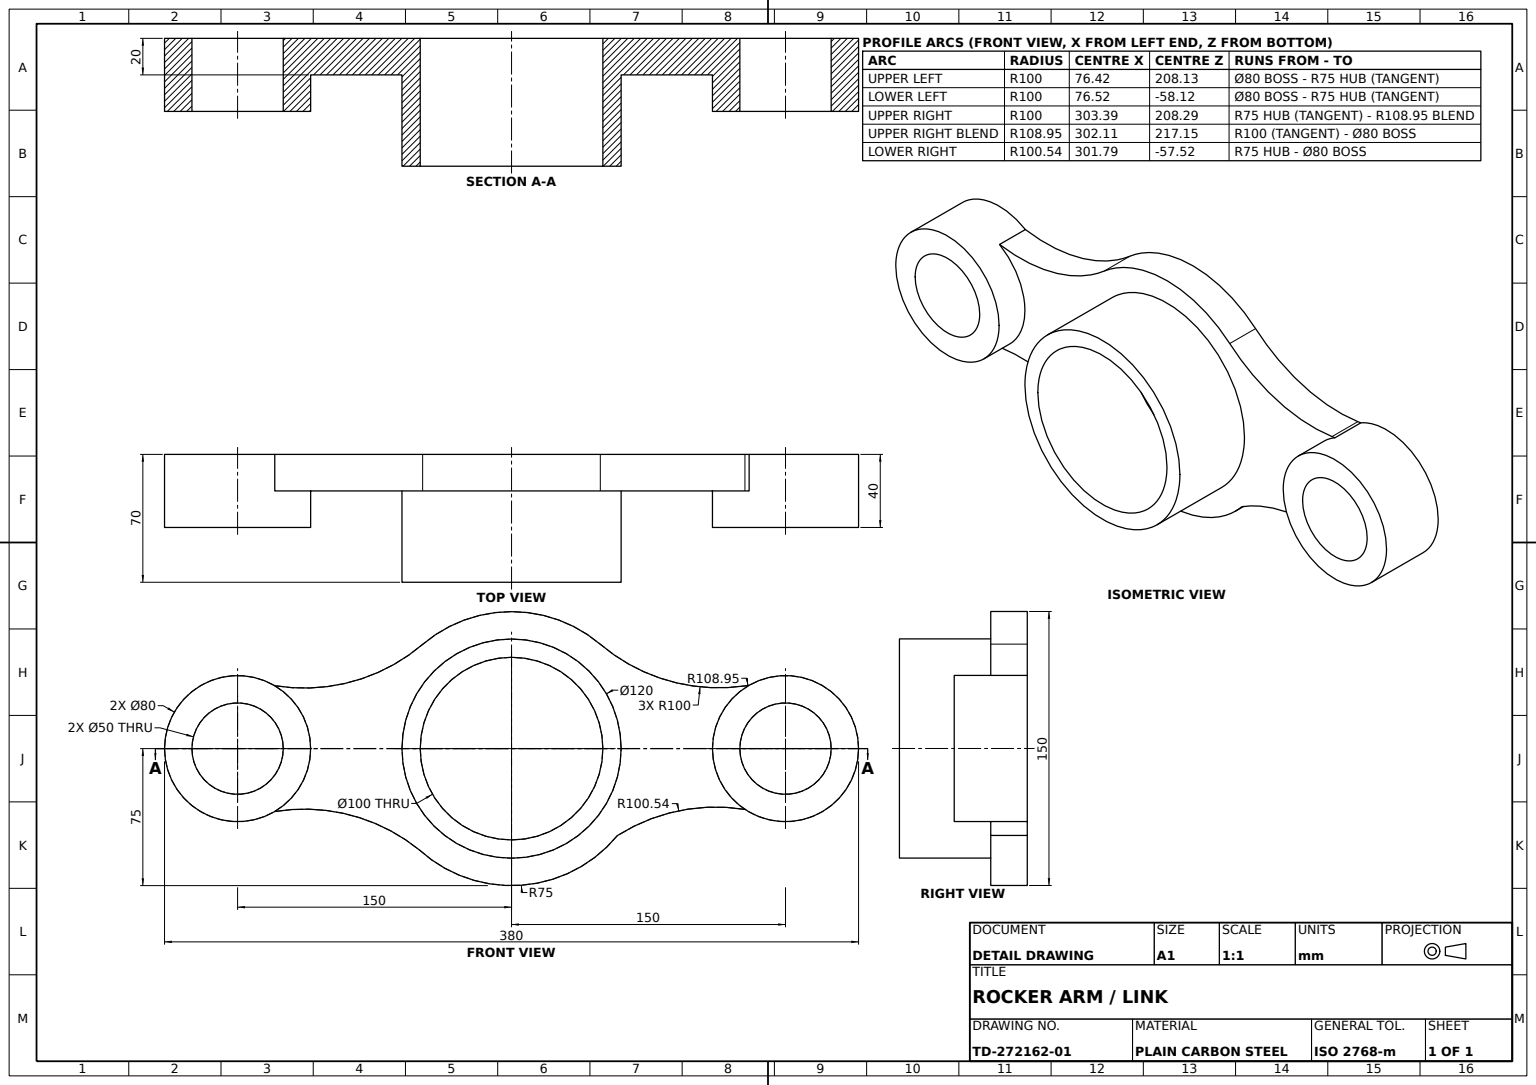
SolidWorks part; units mm, degrees
material "Plain Carbon Steel"
ref_plane "Front Plane" through (0, 0, 0) normal (0, 0, 1) x (1, 0, 0)
ref_plane "Top Plane" through (0, 0, 0) normal (0, 1, 0) x (1, 0, 0)
ref_plane "Right Plane" through (0, 0, 0) normal (1, 0, 0) x (0, 0, -1)
sketch "Link Profile Sketch" plane through (0, 0, 0) normal (0, 0, 1) x (1, 0, 0)
  arc A1 (-129.6423, 34.432) -> (-129.6423, -34.432) centre (-150, 0) ccw
  arc A2 (127.7843, -33.2635) -> (130.0893, 34.6924) centre (150, 0) ccw
  arc A3 (-150, 40) -> (-147.9847, 39.2383) centre (-111.3927, 139.1034) ccw
  arc A4 (-50.5482, -55.4065) -> (57.9498, -47.6111) centre (0, 0) ccw
  arc A5 (127.7843, 34.332) -> (130.0893, 34.6924) centre (112.1066, 142.1518) ccw
  arc A6 (-129.6423, -34.432) -> (-50.5482, -55.4065) centre (-113.4841, -133.1179) cw
  arc A7 (48.5979, 57.1249) -> (-48.6772, 57.0573) centre (0, 0) ccw
  arc A8 (127.7843, 34.332) -> (48.5979, 57.1249) centre (113.395, 133.2913) cw
  arc A9 (-129.6423, 34.432) -> (-48.6772, 57.0573) centre (-113.5801, 133.1336) ccw
  arc A10 (127.7843, -33.2635) -> (57.9498, -47.6111) centre (111.7861, -132.5225) ccw
  arc A11 (48.5979, 57.1249) -> (-48.6772, 57.0573) centre (0, 0) ccw
  point P20 (57.9498, 47.6111)
  dimension "D1" = 150
  dimension "D2" = 80
  dimension "D3" = 80
  dimension "D4" = 100
  dimension "D5" = 100
  dimension "D6" = 100
  dimension "D7" = 40
  dimension "D8" = 106.358
  dimension "D9" = 75
  dimension "D10" = 108.9536
  dimension "D11" = 100.54
  dimension "D12" = 19.9107
  dimension "D13" = 22.2157
  dimension "D14" = 36.605
  dimension "D15" = 198.6772
  dimension "D16" = 200.5482
  dimension "D17" = 261.3927
extrude "Link Plate" add sketch "Link Profile Sketch" along normal blind 20
sketch "Center Boss Sketch" plane through (0, 0, 20) normal (0, 0, 1) x (1, 0, 0)
  circle A0 centre (0, 0) radius 60
  dimension "D1" = 120
  dimension "D2" = 120
extrude "Center Boss Ø120" add sketch "Center Boss Sketch" along normal blind 50
sketch "Center Bore Sketch" plane through (0, 0, 70) normal (0, 0, 1) x (1, 0, 0)
  circle A0 centre (0, 0) radius 50
  dimension "D1" = 100
  dimension "D2" = 100
extrude "Center Bore Ø100" cut sketch "Center Bore Sketch" against normal blind 70
sketch "End Boss A Sketch" plane through (0, 0, 20) normal (0, 0, 1) x (1, 0, 0)
  circle A0 centre (-150, 0) radius 40
  dimension "D1" = 80
  dimension "D2" = 80
extrude "End Boss A Ø80" add sketch "End Boss A Sketch" along normal blind 20
sketch "End Boss B Sketch" plane through (0, 0, 20) normal (0, 0, 1) x (1, 0, 0)
  circle A0 centre (150, 0) radius 40
  dimension "D1" = 80
  dimension "D2" = 80
extrude "End Boss B Ø80" add sketch "End Boss B Sketch" along normal blind 20
sketch "End Bores Sketch" plane through (0, 0, 40) normal (0, 0, 1) x (1, 0, 0)
  circle A0 centre (-150, 0) radius 25
  circle A1 centre (150, 0) radius 25
  dimension "D1" = 50
  dimension "D2" = 50
  dimension "D3" = 50
extrude "End Bores 2xØ50" cut sketch "End Bores Sketch" against normal blind 40
